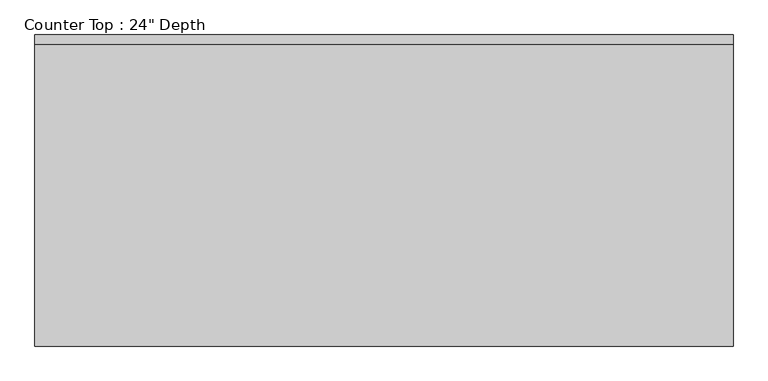
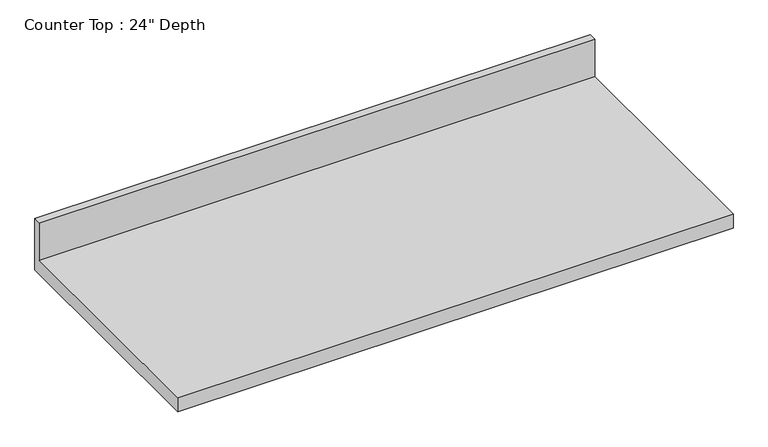
"""IFC4 building model written with IfcOpenShell, lengths in millimetres: furniture geometry."""

from ifc_helpers import new_model, si_unit, frame, origin, place, context, project, spatial, polyline, outline, extrude, source, transform, mapped, element, save


def furniture_03a15ce7(model_context):
    return source(origin(), model_context, "Body", "SweptSolid", [
        extrude(outline(polyline([(0.0, 1016.0), (0.0, 876.3), (-635.0, 876.3), (-635.0, 914.4), (-19.05, 914.4), (-19.05, 1016.0), (0.0, 1016.0)])), frame((-1200.4622951, 0.0, 0.0), z_axis=(1.0, 0.0, 0.0), x_axis=(0.0, 1.0, 0.0)), (0.0, 0.0, 1.0), 1425.0801823),
    ])


if __name__ == "__main__":
    model = new_model("IFC4")
    model_context = context("Model", 3, world=origin())
    ifc_project = project(units=[si_unit("LENGTHUNIT", "METRE", prefix="MILLI")], contexts=[model_context])
    site = spatial("IfcSite", under=ifc_project)
    building = spatial("IfcBuilding", under=site)
    placement = place(None, origin())
    furniture_shape = furniture_03a15ce7(model_context)
    element("IfcFurniture", 1, ObjectType="Counter Top : 24\" Depth", at=placement, inside=building, context=model_context, shape_type="MappedRepresentation", body=[
        mapped(furniture_shape, transform((0.0, 0.0, 0.0), x_axis=(1.0, 0.0, 0.0), y_axis=(0.0, 1.0, 0.0), z_axis=(0.0, 0.0, 1.0))),
    ])
    save(model, "model.ifc")

# Revit data of these elements
# Type "Counter Top : 24\" Depth"
#   Assembly Code = "C1030400"
#   Counter Thickness = 0' - 1 1/2"
#   Depth = 2' - 1"
#   Height = 3' - 0"
#   Length [instance default] = 8' - 0"
#   Counter Top Material = none
#   Default Elevation = 0
# Element 1 (IfcFurniture, "Counter Top : 24\" Depth")
#   Length = 4' - 8.10552"
#   Materials on its faces: "Counter Top"
# Materials
#   "Counter Top": class "Wood", colour RGB 226 177 128, transparency 0
